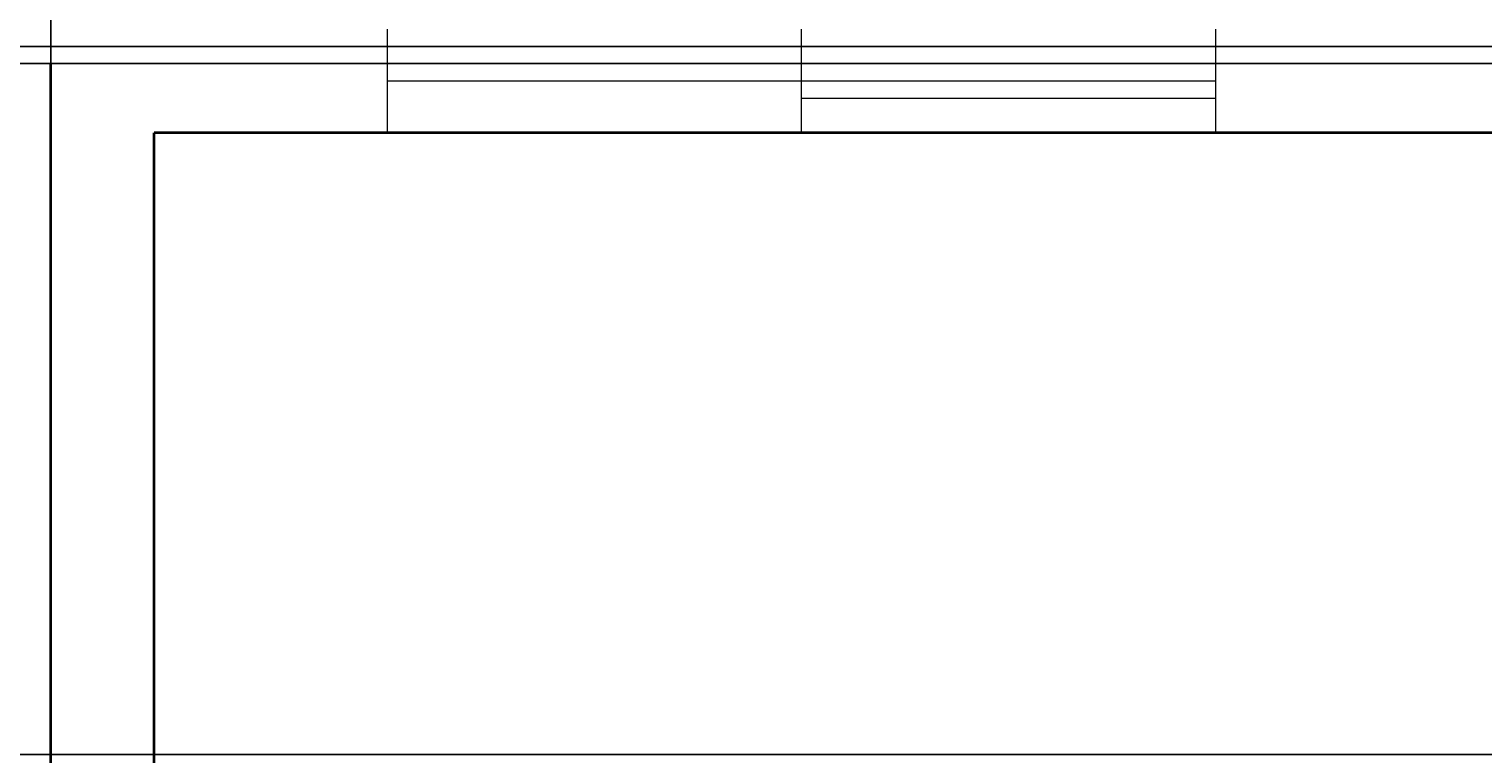
# Model space of a CAD drawing. Units: feet. Extents: x 105 to 1094, y -88 to 588.
# Tile 22 of 59: x 149 to 234, y 354 to 396. Entities that reach past the tile are written whole.
import ezdxf

# ---------------------------------------------------------------- set-up
doc = ezdxf.new("R2010")
doc.units = ezdxf.units.FT
doc.header["$MEASUREMENT"] = 0
for name, color, linetype, lineweight in [('A-ANNO-DIMS', 2, 'Continuous', 18), ('A-FLOR-PROJ', 8, 'Continuous', 25), ('A-GLAZ', 4, 'Continuous', 18), ('A-WALL', 7, 'Continuous', 35)]:
    doc.layers.add(name, color=color, linetype=linetype, lineweight=lineweight)
doc.styles.get("Standard").update_dxf_attribs({"font": 'arial.ttf'})
doc.dimstyles.get("Standard").update_dxf_attribs({"dimtxt": 0.18, "dimasz": 0.18, "dimexe": 0.18, "dimexo": 0.0625, "dimgap": 0.09, "dimtad": 0, "dimtih": 1, "dimtoh": 1, "dimdec": 4, "dimzin": 0, "dimdsep": 46, "dimtxsty": 'Standard', "dimcen": 0.09, "dimadec": 0, "dimazin": 0, "dimtfac": 1, "dimtdec": 4, "dimtofl": 0, "dimtmove": 0, "dimatfit": 3, "dimfxl": 1, "dimtolj": 1, "dimtzin": 0, "dimarcsym": 0})

# ---------------------------------------------------------------- blocks, each defined once
blk = doc.blocks.new('WIN-TWO-LIGHT')
for p, q in [((0, 0), (0, 6)), ((24, 0), (24, 6)), ((48, 0), (48, 6)), ((24, 4), (48, 4)), ((0, 3), (48, 3)), ((0, 2), (24, 2))]:
    blk.add_line(p, q)
blk = doc.blocks.new('*D21')
at = {"layer": 'A-ANNO-DIMS', "color": 0, "lineweight": -2, "transparency": 16777216}
for p, q in [((849.626, 543.081), (105.458, 543.081)), ((105.638, 542.901), (105.638, 250.263)), ((105.638, -42.739), (105.638, 249.899)), ((849.626, -42.919), (105.458, -42.919))]:
    blk.add_line(p, q, dxfattribs=at)
at = {"layer": 'A-ANNO-DIMS', "color": 0, "transparency": 16777216}
for points in [[(105.608, 542.901), (105.668, 542.901), (105.638, 543.081)], [(105.608, -42.739), (105.668, -42.739), (105.638, -42.919)]]:
    blk.add_solid(points, dxfattribs=at)
at = {"layer": 'Defpoints', "color": 0, "transparency": 16777216}
for p in [(105.638, 543.081), (849.688, 543.081), (849.688, -42.919)]:
    blk.add_point(p, dxfattribs=at)
at = {"layer": 'A-ANNO-DIMS', "color": 0, "transparency": 16777216, "insert": (105.638, 250.081), "char_height": 0.18, "attachment_point": 5}
blk.add_mtext('\\A1;586', dxfattribs=at)
blk = doc.blocks.new('*D28')
at = {"layer": 'A-ANNO-DIMS', "color": 0, "lineweight": -2, "transparency": 16777216}
for p, q in [((150.626, 424.081), (105.458, 424.081)), ((105.638, 423.901), (105.638, 350.263)), ((105.638, 276.261), (105.638, 349.899)), ((150.626, 276.081), (105.458, 276.081))]:
    blk.add_line(p, q, dxfattribs=at)
at = {"layer": 'A-ANNO-DIMS', "color": 0, "transparency": 16777216}
for points in [[(105.608, 423.901), (105.668, 423.901), (105.638, 424.081)], [(105.608, 276.261), (105.668, 276.261), (105.638, 276.081)]]:
    blk.add_solid(points, dxfattribs=at)
at = {"layer": 'Defpoints', "color": 0, "transparency": 16777216}
for p in [(105.638, 424.081), (150.688, 424.081), (150.688, 276.081)]:
    blk.add_point(p, dxfattribs=at)
at = {"layer": 'A-ANNO-DIMS', "color": 0, "transparency": 16777216, "insert": (105.638, 350.081), "char_height": 0.18, "attachment_point": 5}
blk.add_mtext('\\A1;148', dxfattribs=at)
blk = doc.blocks.new('*D33')
at = {"layer": 'A-ANNO-DIMS', "color": 0, "lineweight": -2, "transparency": 16777216}
for p, q in [((646.626, 395.081), (105.458, 395.081)), ((105.638, 394.901), (105.638, 345.263)), ((105.638, 295.261), (105.638, 344.899)), ((646.626, 295.081), (105.458, 295.081))]:
    blk.add_line(p, q, dxfattribs=at)
at = {"layer": 'A-ANNO-DIMS', "color": 0, "transparency": 16777216}
for points in [[(105.608, 394.901), (105.668, 394.901), (105.638, 395.081)], [(105.608, 295.261), (105.668, 295.261), (105.638, 295.081)]]:
    blk.add_solid(points, dxfattribs=at)
at = {"layer": 'Defpoints', "color": 0, "transparency": 16777216}
for p in [(646.688, 395.081), (105.638, 295.081), (646.688, 295.081)]:
    blk.add_point(p, dxfattribs=at)
at = {"layer": 'A-ANNO-DIMS', "color": 0, "transparency": 16777216, "insert": (105.638, 345.081), "char_height": 0.18, "attachment_point": 5}
blk.add_mtext('\\A1;100', dxfattribs=at)
blk = doc.blocks.new('*D38')
at = {"layer": 'A-ANNO-DIMS', "color": 0, "lineweight": -2, "transparency": 16777216}
for p, q in [((150.688, 224.144), (150.688, 588.311)), ((150.868, 588.131), (222.408, 588.131)), ((294.508, 588.131), (222.968, 588.131)), ((294.688, 224.144), (294.688, 588.311))]:
    blk.add_line(p, q, dxfattribs=at)
at = {"layer": 'A-ANNO-DIMS', "color": 0, "transparency": 16777216}
for points in [[(150.868, 588.161), (150.868, 588.101), (150.688, 588.131)], [(294.508, 588.161), (294.508, 588.101), (294.688, 588.131)]]:
    blk.add_solid(points, dxfattribs=at)
at = {"layer": 'Defpoints', "color": 0, "transparency": 16777216}
for p in [(294.688, 588.131), (150.688, 224.081), (294.688, 224.081)]:
    blk.add_point(p, dxfattribs=at)
at = {"layer": 'A-ANNO-DIMS', "color": 0, "transparency": 16777216, "insert": (222.688, 588.131), "char_height": 0.18, "attachment_point": 5}
blk.add_mtext('\\A1;144', dxfattribs=at)
blk = doc.blocks.new('*D51')
at = {"layer": 'A-ANNO-DIMS', "color": 0, "lineweight": -2, "transparency": 16777216}
for p, q in [((432.626, 394.081), (105.458, 394.081)), ((105.638, 393.901), (105.638, 374.263)), ((105.638, 354.261), (105.638, 373.899)), ((426.626, 354.081), (105.458, 354.081))]:
    blk.add_line(p, q, dxfattribs=at)
at = {"layer": 'A-ANNO-DIMS', "color": 0, "transparency": 16777216}
for points in [[(105.608, 393.901), (105.668, 393.901), (105.638, 394.081)], [(105.608, 354.261), (105.668, 354.261), (105.638, 354.081)]]:
    blk.add_solid(points, dxfattribs=at)
at = {"layer": 'Defpoints', "color": 0, "transparency": 16777216}
for p in [(432.688, 394.081), (105.638, 354.081), (426.688, 354.081)]:
    blk.add_point(p, dxfattribs=at)
at = {"layer": 'A-ANNO-DIMS', "color": 0, "transparency": 16777216, "insert": (105.638, 374.081), "char_height": 0.18, "attachment_point": 5}
blk.add_mtext('\\A1;40', dxfattribs=at)

msp = doc.modelspace()

# ---------------------------------------------------------------- linework, layer by layer
at = {"layer": 'A-FLOR-PROJ'}
msp.add_line((150.6883, 424.0812), (150.6883, 394.0812), dxfattribs=at)
at = {"layer": 'A-WALL'}
for p, q in [((150.6883, 276.0812), (150.6883, 394.0812)), ((307.6883, 390.0812), (156.6883, 390.0812)), ((156.6883, 282.0812), (156.6883, 390.0812))]:
    msp.add_line(p, q, dxfattribs=at)

# ---------------------------------------------------------------- block references
at = {"layer": 'A-GLAZ', "extrusion": (0, 0, -1), "zscale": -1, "rotation": 180}
msp.add_blockref('WIN-TWO-LIGHT', (-170.188, 396.0813), dxfattribs=at)

# ---------------------------------------------------------------- dimensions: what is measured, and where the dimension line sits
at = {"layer": 'A-ANNO-DIMS'}
dim = msp.add_linear_dim(base=(294.6883, 588.1312), p1=(150.6883, 224.0812), p2=(294.6883, 224.0812), dimstyle='Standard', override={"dimdec": 0, "dimlfac": 1, "dimrnd": 0, "dimzin": 0, "dimdsep": 46, "dimlunit": 2}, dxfattribs=at)
dim.commit()
dim.dimension.update_dxf_attribs({"geometry": '*D38', "text_midpoint": (222.6883, 588.1312)})
for base, p1, p2, picture, middle in [((105.6383, 543.0812), (849.6883, -42.9188), (849.6883, 543.0812), '*D21', (105.6383, 250.0812)), ((105.6383, 424.0812), (150.6883, 276.0812), (150.6883, 424.0812), '*D28', (105.6383, 350.0812)), ((105.6383, 295.0812), (646.6883, 395.0812), (646.6883, 295.0812), '*D33', (105.6383, 345.0812)), ((105.6383, 354.0812), (432.6883, 394.0812), (426.6883, 354.0812), '*D51', (105.6383, 374.0812))]:
    dim = msp.add_linear_dim(base=base, p1=p1, p2=p2, angle=90, dimstyle='Standard', override={"dimdec": 0, "dimlfac": 1, "dimrnd": 0, "dimzin": 0, "dimdsep": 46, "dimlunit": 2}, dxfattribs=at)
    dim.commit()
    dim.dimension.update_dxf_attribs({"geometry": picture, "text_midpoint": middle})

doc.saveas('drawing.dxf')
